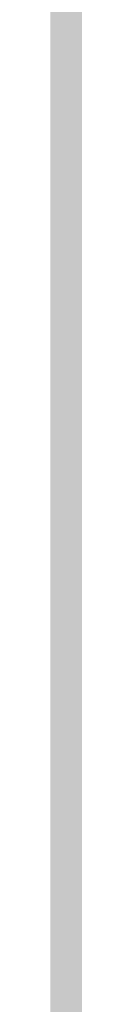
# Model space of a CAD drawing. Units: millimetres. Extents: x 0 to 2267, y 0 to 1823.
# Tile 40 of 256: x 1593.4301 to 1593.4369, y 1226.3857 to 1226.718. Entities that reach past the tile are written whole.
import ezdxf

# ---------------------------------------------------------------- set-up
doc = ezdxf.new("R2010")
doc.units = ezdxf.units.MM
doc.header["$MEASUREMENT"] = 0
doc.layers.add('M-HATC', color=252, linetype='Continuous', lineweight=18)

msp = doc.modelspace()

# ---------------------------------------------------------------- hatches: boundary and pattern name
at = {"layer": 'M-HATC'}
h = msp.add_hatch(color=256, dxfattribs=at)
h.dxf.hatch_style = 1
h.paths.add_polyline_path([(2055.77105, 1603.06204), (1381.08677, 1603.06204), (1381.08677, 1598.06204), (2055.77105, 1598.06204)])
h.paths.add_polyline_path([(2055.77105, 1598.06204), (1381.08677, 1598.06204), (1381.08677, 1593.06204), (2055.77105, 1593.06204)])
h.paths.add_polyline_path([(2051.30737, 1536.76088), (1385.55044, 1536.76088), (1385.55044, 1526.76088), (1387.55044, 1526.76088), (1388.53662, 1525.05276), (1385.33187, 1521.23348), (1385.33187, 1521.22256), (2050.25417, 1522.74913), (2048.32119, 1525.05276), (2049.30737, 1526.76088), (2051.30737, 1526.76088)])
edge = h.paths.add_edge_path()
edge.add_arc((1847.53451, 1379.14917), 135, 222.6030607, 222.8908505, ccw=False)
edge.add_line((1748.16629, 1287.76561), (1683.09212, 1287.76561))
edge.add_arc((1583.7239, 1379.14917), 135, 317.1091495, 317.3969393, ccw=False)
edge.add_arc((1678.9686, 1290.67067), 5, 222.89085, 317.10915, ccw=False)
edge.add_arc((1774.21331, 1379.14917), 135, 222.6030607, 222.8908505, ccw=False)
edge.add_line((1674.84509, 1287.76561), (1609.77092, 1287.76561))
edge.add_arc((1510.4027, 1379.14917), 135, 317.1091495, 317.3969393, ccw=False)
edge.add_arc((1605.6474, 1290.67067), 5, 222.89085, 317.10915, ccw=False)
edge.add_arc((1700.89211, 1379.14917), 135, 222.6030607, 222.8908505, ccw=False)
edge.add_line((1601.52388, 1287.76561), (1536.44972, 1287.76561))
edge.add_arc((1437.08149, 1379.14917), 135, 317.1091495, 317.3969393, ccw=False)
edge.add_arc((1532.3262, 1290.67067), 5, 222.89085, 317.10915, ccw=False)
edge.add_arc((1627.57091, 1379.14917), 135, 222.6030607, 222.8908505, ccw=False)
edge.add_line((1528.20268, 1287.76561), (1505.92891, 1287.76561))
edge.add_spline(control_points=[(1505.92891, 1287.76561), (1504.26224, 1287.76561), (1504.26224, 1282.76561), (1505.92891, 1282.76561)], knot_values=[0, 0, 0, 0, 5, 5, 5, 5], degree=3, periodic=0)
edge.add_line((1505.92891, 1282.76561), (1930.92891, 1282.76561))
edge.add_spline(control_points=[(1930.92891, 1282.76561), (1932.59557, 1282.76561), (1932.59557, 1287.76561), (1930.92891, 1287.76561)], knot_values=[0, 0, 0, 0, 5, 5, 5, 5], degree=3, periodic=0)
edge.add_line((1930.92891, 1287.76561), (1903.05573, 1287.76561))
edge.add_arc((1803.6875, 1379.14917), 135, 317.1091495, 317.3969393, ccw=False)
edge.add_arc((1898.93221, 1290.67067), 5, 222.89085, 317.10915, ccw=False)
edge.add_arc((1994.17691, 1379.14917), 135, 222.6030607, 222.8908505, ccw=False)
edge.add_line((1894.80869, 1287.76561), (1829.73452, 1287.76561))
edge.add_arc((1730.3663, 1379.14917), 135, 317.1091495, 317.3969393, ccw=False)
edge.add_arc((1825.61101, 1290.67067), 5, 222.89085, 317.10915, ccw=False)
edge.add_arc((1920.85571, 1379.14917), 135, 222.6030607, 222.8908505, ccw=False)
edge.add_line((1821.48749, 1287.76561), (1756.41332, 1287.76561))
edge.add_arc((1657.0451, 1379.14917), 135, 317.1091495, 317.3969393, ccw=False)
edge.add_arc((1752.28981, 1290.67067), 5, 222.89085, 317.10915, ccw=False)
edge = h.paths.add_edge_path()
edge.add_spline(control_points=[(1843.42891, 1227.24746), (1845.09557, 1227.24746), (1845.09557, 1232.24746), (1843.42891, 1232.24746)], knot_values=[0, 0, 0, 0, 5, 5, 5, 5], degree=3, periodic=0)
edge.add_line((1843.42891, 1232.24746), (1593.42891, 1232.24746))
edge.add_spline(control_points=[(1593.42891, 1232.24746), (1591.76224, 1232.24746), (1591.76224, 1227.24746), (1593.42891, 1227.24746)], knot_values=[0, 0, 0, 0, 5, 5, 5, 5], degree=3, periodic=0)
edge.add_line((1593.42891, 1227.24746), (1843.42891, 1227.24746))
h.paths.add_polyline_path([(1905.92891, 1127.41706), (1530.92891, 1127.41706, 0.414214), (1520.92891, 1117.41706), (1530.92891, 1117.41706), (1915.92891, 1117.41706, 0.414214)])
edge = h.paths.add_edge_path()
edge.add_arc((1397.08577, 1498.40775), 12.72993, 90.782146, 190.878706, ccw=False)
edge.add_line((1396.912, 1511.13649), (1428.00968, 1511.34875))
edge.add_line((1428.00968, 1511.34875), (1433.00968, 1511.34875))
edge.add_line((1433.00968, 1511.34875), (1434.439, 1511.34875))
edge.add_arc((1419.474, 1498.08041), 20, 41.560995, 74.082109)
edge.add_line((1424.95919, 1517.31353), (1399.93509, 1517.25608))
edge.add_spline(control_points=[(1399.93074, 1517.25607), (1399.88398, 1517.21312), (1399.8328, 1517.16893), (1399.77741, 1517.1236)], knot_values=[11.567499, 11.567499, 11.567499, 11.567499, 11.814249, 11.814249, 11.814249, 11.814249], degree=3, periodic=0)
edge.add_spline(control_points=[(1399.63279, 1517.00986), (1399.58305, 1516.97214), (1399.53072, 1516.93375), (1399.47591, 1516.89474)], knot_values=[11.167718, 11.167718, 11.167718, 11.167718, 11.365188, 11.365188, 11.365188, 11.365188], degree=3, periodic=0)
edge.add_spline(control_points=[(1399.33981, 1516.80007), (1399.15144, 1516.67185), (1398.93836, 1516.5377), (1398.70404, 1516.39942)], knot_values=[10.376405, 10.376405, 10.376405, 10.376405, 11.00994, 11.00994, 11.00994, 11.00994], degree=3, periodic=0)
edge.add_spline(control_points=[(1398.65716, 1516.37187), (1398.57885, 1516.32602), (1398.49825, 1516.27974), (1398.41549, 1516.23309)], knot_values=[10.125175, 10.125175, 10.125175, 10.125175, 10.334406, 10.334406, 10.334406, 10.334406], degree=3, periodic=0)
edge.add_spline(control_points=[(1398.26422, 1516.14874), (1398.19595, 1516.11107), (1398.12634, 1516.07319), (1398.05546, 1516.03513)], knot_values=[9.832246, 9.832246, 9.832246, 9.832246, 9.999658, 9.999658, 9.999658, 9.999658], degree=3, periodic=0)
edge.add_spline(control_points=[(1397.9987, 1516.00476), (1397.73115, 1515.86211), (1397.44602, 1515.71707), (1397.14664, 1515.57138)], knot_values=[9.161808, 9.161808, 9.161808, 9.161808, 9.787769, 9.787769, 9.787769, 9.787769], degree=3, periodic=0)
edge.add_spline(control_points=[(1397.14664, 1515.57138), (1396.84182, 1515.42305), (1396.52223, 1515.27404), (1396.1914, 1515.12621)], knot_values=[8.524455, 8.524455, 8.524455, 8.524455, 9.161808, 9.161808, 9.161808, 9.161808], degree=3, periodic=0)
edge.add_spline(control_points=[(1396.07771, 1515.07565), (1395.98538, 1515.03478), (1395.89222, 1514.99402), (1395.7983, 1514.9534)], knot_values=[8.275193, 8.275193, 8.275193, 8.275193, 8.451726, 8.451726, 8.451726, 8.451726], degree=3, periodic=0)
edge.add_spline(control_points=[(1395.60184, 1514.86912), (1395.49975, 1514.82568), (1395.39685, 1514.78244), (1395.29322, 1514.73944)], knot_values=[7.962917, 7.962917, 7.962917, 7.962917, 8.152764, 8.152764, 8.152764, 8.152764], degree=3, periodic=0)
edge.add_spline(control_points=[(1395.21158, 1514.70568), (1394.82779, 1514.5475), (1394.43452, 1514.39287), (1394.03645, 1514.24422)], knot_values=[7.21254, 7.21254, 7.21254, 7.21254, 7.913148, 7.913148, 7.913148, 7.913148], degree=3, periodic=0)
edge.add_spline(control_points=[(1394.03645, 1514.24422), (1393.70758, 1514.12142), (1393.37544, 1514.0027), (1393.04267, 1513.88945)], knot_values=[6.633733, 6.633733, 6.633733, 6.633733, 7.21254, 7.21254, 7.21254, 7.21254], degree=3, periodic=0)
edge.add_spline(control_points=[(1392.82142, 1513.81499), (1392.71978, 1513.78118), (1392.61815, 1513.74791), (1392.51658, 1513.71521)], knot_values=[6.328796, 6.328796, 6.328796, 6.328796, 6.505493, 6.505493, 6.505493, 6.505493], degree=3, periodic=0)
edge.add_spline(control_points=[(1392.51658, 1513.71521), (1392.31873, 1513.65151), (1392.12116, 1513.59001), (1391.92441, 1513.53098)], knot_values=[5.984605, 5.984605, 5.984605, 5.984605, 6.328796, 6.328796, 6.328796, 6.328796], degree=3, periodic=0)
edge.add_spline(control_points=[(1391.79155, 1513.49146), (1391.31215, 1513.35011), (1390.83842, 1513.22392), (1390.37844, 1513.11711)], knot_values=[5.066697, 5.066697, 5.066697, 5.066697, 5.907055, 5.907055, 5.907055, 5.907055], degree=3, periodic=0)
edge.add_spline(control_points=[(1390.37844, 1513.11711), (1390.17973, 1513.07097), (1389.98359, 1513.02845), (1389.79067, 1512.98988)], knot_values=[4.70367, 4.70367, 4.70367, 4.70367, 5.066695, 5.066695, 5.066695, 5.066695], degree=3, periodic=0)
edge.add_spline(control_points=[(1389.42203, 1512.92036), (1389.24588, 1512.88922), (1389.0729, 1512.86172), (1388.90364, 1512.83814)], knot_values=[4.130571, 4.130571, 4.130571, 4.130571, 4.469816, 4.469816, 4.469816, 4.469816], degree=3, periodic=0)
edge.add_spline(control_points=[(1388.90364, 1512.83814), (1388.59103, 1512.7946), (1388.29108, 1512.76444), (1388.00714, 1512.74941)], knot_values=[3.504031, 3.504031, 3.504031, 3.504031, 4.130571, 4.130571, 4.130571, 4.130571], degree=3, periodic=0)
edge.add_spline(control_points=[(1387.9356, 1512.74593), (1387.85378, 1512.74231), (1387.77334, 1512.73997), (1387.69435, 1512.73898)], knot_values=[3.268866, 3.268866, 3.268866, 3.268866, 3.451164, 3.451164, 3.451164, 3.451164], degree=3, periodic=0)
edge.add_spline(control_points=[(1387.33512, 1512.74426), (1387.20757, 1512.74991), (1387.08472, 1512.7597), (1386.96699, 1512.77385)], knot_values=[2.670686, 2.670686, 2.670686, 2.670686, 2.984, 2.984, 2.984, 2.984], degree=3, periodic=0)
edge.add_spline(control_points=[(1386.83274, 1512.79225), (1386.82093, 1512.79407), (1386.80917, 1512.79594), (1386.79747, 1512.79787)], knot_values=[2.516981, 2.516981, 2.516981, 2.516981, 2.549528, 2.549528, 2.549528, 2.549528], degree=3, periodic=0)
edge.add_spline(control_points=[(1386.45257, 1512.87348), (1386.42573, 1512.88105), (1386.39931, 1512.88895), (1386.3733, 1512.89719)], knot_values=[2.095869, 2.095869, 2.095869, 2.095869, 2.17941, 2.17941, 2.17941, 2.17941], degree=3, periodic=0)
edge.add_spline(control_points=[(1386.06911, 1513.01889), (1386.06338, 1513.02174), (1386.05768, 1513.02463), (1386.05201, 1513.02753)], knot_values=[1.72453, 1.72453, 1.72453, 1.72453, 1.745933, 1.745933, 1.745933, 1.745933], degree=3, periodic=0)
edge.add_arc((1399.474, 1498.08041), 20, 131.824322, 180)
edge.add_arc((1630.33362, 1505.54843), 250.97076, 181.7051759, 236.427975)
edge.add_arc((1605.33992, 1483.30441), 218.7822, 238.660829, 243.3496099)
edge.add_arc((1647.09105, 1510.35917), 262.89859, 183.1298361, 237.8534422, ccw=False)
h.paths.add_polyline_path([(1406.53685, 1391.96444, 0.149382), (1491.55061, 1296.44177, -0.129517)], flags=17)
edge = h.paths.add_edge_path()
edge.add_arc((2037.38381, 1498.08041), 20, 0, 48.265868)
edge.add_spline(control_points=[(2050.69731, 1513.00525), (2050.65121, 1512.98471), (2050.60338, 1512.96554), (2050.55388, 1512.94771)], knot_values=[1.835652, 1.835652, 1.835652, 1.835652, 2.000781, 2.000781, 2.000781, 2.000781], degree=3, periodic=0)
edge.add_spline(control_points=[(2050.46156, 1512.91661), (2050.479, 1512.9221), (2050.49625, 1512.92774), (2050.51332, 1512.93353)], knot_values=[2.045477, 2.045477, 2.045477, 2.045477, 2.101389, 2.101389, 2.101389, 2.101389], degree=3, periodic=0)
edge.add_spline(control_points=[(2050.12896, 1512.83416), (2050.19843, 1512.84734), (2050.26573, 1512.86233), (2050.33075, 1512.87919)], knot_values=[2.237629, 2.237629, 2.237629, 2.237629, 2.435841, 2.435841, 2.435841, 2.435841], degree=3, periodic=0)
edge.add_spline(control_points=[(2050.09463, 1512.82783), (2050.10613, 1512.82989), (2050.11757, 1512.832), (2050.12896, 1512.83416)], knot_values=[2.435841, 2.435841, 2.435841, 2.435841, 2.468321, 2.468321, 2.468321, 2.468321], degree=3, periodic=0)
edge.add_spline(control_points=[(2049.78433, 1512.78511), (2049.85521, 1512.79219), (2049.92435, 1512.80077), (2049.99166, 1512.81088)], knot_values=[2.563852, 2.563852, 2.563852, 2.563852, 2.748541, 2.748541, 2.748541, 2.748541], degree=3, periodic=0)
edge.add_spline(control_points=[(2049.4052, 1512.76169), (2049.5364, 1512.76526), (2049.66292, 1512.77299), (2049.78433, 1512.78511)], knot_values=[2.748541, 2.748541, 2.748541, 2.748541, 3.064882, 3.064882, 3.064882, 3.064882], degree=3, periodic=0)
edge.add_spline(control_points=[(2049.16976, 1512.75968), (2049.23364, 1512.7591), (2049.29654, 1512.7594), (2049.35844, 1512.7606)], knot_values=[3.102309, 3.102309, 3.102309, 3.102309, 3.2503, 3.2503, 3.2503, 3.2503], degree=3, periodic=0)
edge.add_spline(control_points=[(2048.85727, 1512.76911), (2048.96378, 1512.76378), (2049.068, 1512.76061), (2049.16976, 1512.75968)], knot_values=[3.2503, 3.2503, 3.2503, 3.2503, 3.486069, 3.486069, 3.486069, 3.486069], degree=3, periodic=0)
edge.add_spline(control_points=[(2048.69241, 1512.77892), (2048.3729, 1512.80093), (2048.0345, 1512.84106), (2047.68175, 1512.89697)], knot_values=[3.606429, 3.606429, 3.606429, 3.606429, 4.2989, 4.2989, 4.2989, 4.2989], degree=3, periodic=0)
edge.add_spline(control_points=[(2047.68175, 1512.89697), (2047.5458, 1512.91852), (2047.40772, 1512.94241), (2047.26776, 1512.96851)], knot_values=[4.2989, 4.2989, 4.2989, 4.2989, 4.565769, 4.565769, 4.565769, 4.565769], degree=3, periodic=0)
edge.add_spline(control_points=[(2047.26776, 1512.96851), (2047.14494, 1512.99141), (2047.02067, 1513.01601), (2046.89514, 1513.04223)], knot_values=[4.565769, 4.565769, 4.565769, 4.565769, 4.799971, 4.799971, 4.799971, 4.799971], degree=3, periodic=0)
edge.add_spline(control_points=[(2046.89514, 1513.04223), (2046.52865, 1513.11875), (2046.15135, 1513.20899), (2045.7676, 1513.31068)], knot_values=[4.799971, 4.799971, 4.799971, 4.799971, 5.483718, 5.483718, 5.483718, 5.483718], degree=3, periodic=0)
edge.add_spline(control_points=[(2045.7676, 1513.31068), (2045.3724, 1513.41539), (2044.97036, 1513.53225), (2044.56625, 1513.65876)], knot_values=[5.483718, 5.483718, 5.483718, 5.483718, 6.187866, 6.187866, 6.187866, 6.187866], degree=3, periodic=0)
edge.add_spline(control_points=[(2044.56625, 1513.65876), (2044.41491, 1513.70614), (2044.26329, 1513.75487), (2044.11163, 1513.80482)], knot_values=[6.187866, 6.187866, 6.187866, 6.187866, 6.451551, 6.451551, 6.451551, 6.451551], degree=3, periodic=0)
edge.add_spline(control_points=[(2044.11163, 1513.80482), (2043.99666, 1513.84269), (2043.88167, 1513.88126), (2043.76676, 1513.92048)], knot_values=[6.451551, 6.451551, 6.451551, 6.451551, 6.651434, 6.651434, 6.651434, 6.651434], degree=3, periodic=0)
edge.add_spline(control_points=[(2043.76676, 1513.92048), (2043.37157, 1514.05536), (2042.97738, 1514.19789), (2042.58863, 1514.34575)], knot_values=[6.651434, 6.651434, 6.651434, 6.651434, 7.338879, 7.338879, 7.338879, 7.338879], degree=3, periodic=0)
edge.add_spline(control_points=[(2042.58863, 1514.34575), (2042.16431, 1514.50715), (2041.74647, 1514.67491), (2041.34086, 1514.84603)], knot_values=[7.338879, 7.338879, 7.338879, 7.338879, 8.089209, 8.089209, 8.089209, 8.089209], degree=3, periodic=0)
edge.add_spline(control_points=[(2041.34086, 1514.84603), (2041.1028, 1514.94647), (2040.86896, 1515.04806), (2040.64049, 1515.1502)], knot_values=[8.089209, 8.089209, 8.089209, 8.089209, 8.529587, 8.529587, 8.529587, 8.529587], degree=3, periodic=0)
edge.add_spline(control_points=[(2040.50999, 1515.20887), (2040.08238, 1515.40218), (2039.67475, 1515.59705), (2039.29495, 1515.78939)], knot_values=[8.613818, 8.613818, 8.613818, 8.613818, 9.44571, 9.44571, 9.44571, 9.44571], degree=3, periodic=0)
edge.add_spline(control_points=[(2039.29495, 1515.78939), (2039.0618, 1515.90746), (2038.83914, 1516.02458), (2038.62878, 1516.1398)], knot_values=[9.44571, 9.44571, 9.44571, 9.44571, 9.956404, 9.956404, 9.956404, 9.956404], degree=3, periodic=0)
edge.add_spline(control_points=[(2038.62878, 1516.1398), (2038.51874, 1516.20007), (2038.41207, 1516.25982), (2038.30903, 1516.31891)], knot_values=[9.956404, 9.956404, 9.956404, 9.956404, 10.223542, 10.223542, 10.223542, 10.223542], degree=3, periodic=0)
edge.add_spline(control_points=[(2038.30903, 1516.31891), (2038.21377, 1516.37354), (2038.12161, 1516.42762), (2038.03275, 1516.48102)], knot_values=[10.223542, 10.223542, 10.223542, 10.223542, 10.47051, 10.47051, 10.47051, 10.47051], degree=3, periodic=0)
edge.add_spline(control_points=[(2038.03275, 1516.48102), (2037.78552, 1516.62961), (2037.56388, 1516.77304), (2037.37225, 1516.909)], knot_values=[10.47051, 10.47051, 10.47051, 10.47051, 11.15767, 11.15767, 11.15767, 11.15767], degree=3, periodic=0)
edge.add_spline(control_points=[(2037.37225, 1516.909), (2037.27893, 1516.9752), (2037.19274, 1517.03963), (2037.11417, 1517.10203)], knot_values=[11.15767, 11.15767, 11.15767, 11.15767, 11.49227, 11.49227, 11.49227, 11.49227], degree=3, periodic=0)
edge.add_spline(control_points=[(2036.85638, 1517.32585), (2036.91481, 1517.26923), (2036.98143, 1517.21027), (2037.05573, 1517.14922)], knot_values=[11.577341, 11.577341, 11.577341, 11.577341, 11.91035, 11.91035, 11.91035, 11.91035], degree=3, periodic=0)
edge.add_spline(control_points=[(2036.80739, 1517.37475), (2036.82301, 1517.35865), (2036.83935, 1517.34235), (2036.85638, 1517.32585)], knot_values=[11.91035, 11.91035, 11.91035, 11.91035, 12.007402, 12.007402, 12.007402, 12.007402], degree=3, periodic=0)
edge.add_spline(control_points=[(2036.70167, 1517.494), (2036.71042, 1517.48299), (2036.71958, 1517.47185), (2036.72913, 1517.4606)], knot_values=[12.184155, 12.184155, 12.184155, 12.184155, 12.255409, 12.255409, 12.255409, 12.255409], degree=3, periodic=0)
edge.add_spline(control_points=[(2036.6159, 1517.6205), (2036.61998, 1517.61304), (2036.6243, 1517.6055), (2036.62885, 1517.59789)], knot_values=[12.487913, 12.487913, 12.487913, 12.487913, 12.541035, 12.541035, 12.541035, 12.541035], degree=3, periodic=0)
edge.add_spline(control_points=[(2036.56349, 1517.78599), (2036.56372, 1517.77936), (2036.56423, 1517.77264), (2036.56502, 1517.76582)], knot_values=[12.911761, 12.911761, 12.911761, 12.911761, 12.968286, 12.968286, 12.968286, 12.968286], degree=3, periodic=0)
edge.add_spline(control_points=[(2036.61663, 1517.93042), (2036.61248, 1517.92586), (2036.60857, 1517.92121), (2036.60491, 1517.91648)], knot_values=[13.382527, 13.382527, 13.382527, 13.382527, 13.433791, 13.433791, 13.433791, 13.433791], degree=3, periodic=0)
edge.add_spline(control_points=[(2036.74902, 1518.01695), (2036.73613, 1518.0116), (2036.72393, 1518.00601), (2036.71242, 1518.00018)], knot_values=[13.726299, 13.726299, 13.726299, 13.726299, 13.809928, 13.809928, 13.809928, 13.809928], degree=3, periodic=0)
edge.add_spline(control_points=[(2036.86043, 1518.05285), (2036.83863, 1518.04743), (2036.81809, 1518.04156), (2036.79879, 1518.03526)], knot_values=[13.910887, 13.910887, 13.910887, 13.910887, 14.02153, 14.02153, 14.02153, 14.02153], degree=3, periodic=0)
edge.add_line((2036.96387, 1518.08041), (2032.38381, 1518.08041))
edge.add_line((2032.38381, 1518.08041), (2027.38381, 1518.08041))
edge.add_line((2027.38381, 1518.08041), (2022.38381, 1518.08041))
edge.add_line((2022.38381, 1518.08041), (2017.38381, 1518.08041))
edge.add_arc((2017.38381, 1498.08041), 20, 90, 138.439005)
edge.add_line((2002.41881, 1511.34875), (2003.84813, 1511.34875))
edge.add_line((2003.84813, 1511.34875), (2008.84813, 1511.34875))
edge.add_line((2008.84813, 1511.34875), (2039.77204, 1511.13768))
edge.add_arc((2039.77204, 1498.40775), 12.72993, -10.878706, 90, ccw=False)
edge.add_arc((1789.76676, 1510.35917), 262.89859, 302.1465578, 356.8701639, ccw=False)
edge.add_arc((1831.51789, 1483.30441), 218.7822, 296.6503901, 301.339171)
edge.add_arc((1806.52419, 1505.54843), 250.97076, 303.572025, 358.2948241)
h.paths.add_polyline_path([(2030.32096, 1391.96444, -0.129517), (1945.3072, 1296.44177, 0.149382)], flags=17)
edge = h.paths.add_edge_path()
edge.add_spline(control_points=[(2037.2464, 1518.08209), (2037.28977, 1518.08098), (2037.33555, 1518.08041), (2037.3838, 1518.08041)], knot_values=[0.000012, 0.000012, 0.000012, 0.000012, 0.144754, 0.144754, 0.144754, 0.144754], degree=3, periodic=0)
edge.add_line((2037.33571, 1518.08041), (2037.00963, 1518.08041))
edge.add_spline(control_points=[(2037.00963, 1518.08041), (2036.98217, 1518.07678), (2036.95605, 1518.07266), (2036.93124, 1518.06808)], knot_values=[14.13465, 14.13465, 14.13465, 14.13465, 14.247197, 14.247197, 14.247197, 14.247197], degree=3, periodic=0)
edge.add_spline(control_points=[(2036.93124, 1518.06808), (2036.92764, 1518.06741), (2036.92407, 1518.06674), (2036.92053, 1518.06605)], knot_values=[14.118315, 14.118315, 14.118315, 14.118315, 14.13465, 14.13465, 14.13465, 14.13465], degree=3, periodic=0)
edge.add_spline(control_points=[(2036.92053, 1518.06605), (2036.9118, 1518.06436), (2036.90323, 1518.06262), (2036.89484, 1518.06081)], knot_values=[14.078086, 14.078086, 14.078086, 14.078086, 14.118315, 14.118315, 14.118315, 14.118315], degree=3, periodic=0)
edge.add_spline(control_points=[(2036.89484, 1518.06081), (2036.88304, 1518.05827), (2036.87157, 1518.05562), (2036.86043, 1518.05285)], knot_values=[14.02153, 14.02153, 14.02153, 14.02153, 14.078086, 14.078086, 14.078086, 14.078086], degree=3, periodic=0)
edge.add_spline(control_points=[(2036.86043, 1518.05285), (2036.83863, 1518.04743), (2036.81809, 1518.04156), (2036.79879, 1518.03526)], knot_values=[13.910887, 13.910887, 13.910887, 13.910887, 14.02153, 14.02153, 14.02153, 14.02153], degree=3, periodic=0)
edge.add_spline(control_points=[(2036.79879, 1518.03526), (2036.79809, 1518.03504), (2036.7974, 1518.03481), (2036.79671, 1518.03458)], knot_values=[13.906906, 13.906906, 13.906906, 13.906906, 13.910887, 13.910887, 13.910887, 13.910887], degree=3, periodic=0)
edge.add_spline(control_points=[(2036.79671, 1518.03458), (2036.78819, 1518.03178), (2036.77991, 1518.02888), (2036.77187, 1518.02591)], knot_values=[13.857826, 13.857826, 13.857826, 13.857826, 13.906906, 13.906906, 13.906906, 13.906906], degree=3, periodic=0)
edge.add_spline(control_points=[(2036.77187, 1518.02591), (2036.76402, 1518.023), (2036.75641, 1518.02002), (2036.74902, 1518.01695)], knot_values=[13.809928, 13.809928, 13.809928, 13.809928, 13.857826, 13.857826, 13.857826, 13.857826], degree=3, periodic=0)
edge.add_spline(control_points=[(2036.74902, 1518.01695), (2036.73613, 1518.0116), (2036.72393, 1518.00601), (2036.71242, 1518.00018)], knot_values=[13.726299, 13.726299, 13.726299, 13.726299, 13.809928, 13.809928, 13.809928, 13.809928], degree=3, periodic=0)
edge.add_spline(control_points=[(2036.71242, 1518.00018), (2036.71211, 1518.00002), (2036.71179, 1517.99986), (2036.71147, 1517.99969)], knot_values=[13.723993, 13.723993, 13.723993, 13.723993, 13.726299, 13.726299, 13.726299, 13.726299], degree=3, periodic=0)
edge.add_spline(control_points=[(2036.71147, 1517.99969), (2036.70634, 1517.99708), (2036.70134, 1517.99441), (2036.69648, 1517.9917)], knot_values=[13.686536, 13.686536, 13.686536, 13.686536, 13.723993, 13.723993, 13.723993, 13.723993], degree=3, periodic=0)
edge.add_spline(control_points=[(2036.69648, 1517.9917), (2036.6919, 1517.98914), (2036.68744, 1517.98654), (2036.6831, 1517.9839)], knot_values=[13.651251, 13.651251, 13.651251, 13.651251, 13.686536, 13.686536, 13.686536, 13.686536], degree=3, periodic=0)
edge.add_spline(control_points=[(2036.6831, 1517.9839), (2036.67641, 1517.97983), (2036.67001, 1517.97566), (2036.6639, 1517.97139)], knot_values=[13.596804, 13.596804, 13.596804, 13.596804, 13.651251, 13.651251, 13.651251, 13.651251], degree=3, periodic=0)
edge.add_spline(control_points=[(2036.6639, 1517.97139), (2036.66358, 1517.97117), (2036.66326, 1517.97094), (2036.66294, 1517.97072)], knot_values=[13.593956, 13.593956, 13.593956, 13.593956, 13.596804, 13.596804, 13.596804, 13.596804], degree=3, periodic=0)
edge.add_spline(control_points=[(2036.66294, 1517.97072), (2036.6603, 1517.96886), (2036.65771, 1517.96698), (2036.65518, 1517.96509)], knot_values=[13.570322, 13.570322, 13.570322, 13.570322, 13.593956, 13.593956, 13.593956, 13.593956], degree=3, periodic=0)
edge.add_spline(control_points=[(2036.65518, 1517.96509), (2036.65251, 1517.9631), (2036.64991, 1517.96108), (2036.64737, 1517.95905)], knot_values=[13.545477, 13.545477, 13.545477, 13.545477, 13.570322, 13.570322, 13.570322, 13.570322], degree=3, periodic=0)
edge.add_spline(control_points=[(2036.64737, 1517.95905), (2036.64721, 1517.95892), (2036.64705, 1517.9588), (2036.64689, 1517.95867)], knot_values=[13.543931, 13.543931, 13.543931, 13.543931, 13.545477, 13.545477, 13.545477, 13.545477], degree=3, periodic=0)
edge.add_spline(control_points=[(2036.64689, 1517.95867), (2036.64121, 1517.95411), (2036.63582, 1517.94945), (2036.63073, 1517.94468)], knot_values=[13.488237, 13.488237, 13.488237, 13.488237, 13.543931, 13.543931, 13.543931, 13.543931], degree=3, periodic=0)
edge.add_spline(control_points=[(2036.63073, 1517.94468), (2036.62817, 1517.94229), (2036.62569, 1517.93988), (2036.62329, 1517.93744)], knot_values=[13.460307, 13.460307, 13.460307, 13.460307, 13.488237, 13.488237, 13.488237, 13.488237], degree=3, periodic=0)
edge.add_spline(control_points=[(2036.62329, 1517.93744), (2036.62151, 1517.93564), (2036.61978, 1517.93383), (2036.61809, 1517.932)], knot_values=[13.439712, 13.439712, 13.439712, 13.439712, 13.460307, 13.460307, 13.460307, 13.460307], degree=3, periodic=0)
edge.add_spline(control_points=[(2036.61809, 1517.932), (2036.6176, 1517.93147), (2036.61711, 1517.93095), (2036.61663, 1517.93042)], knot_values=[13.433791, 13.433791, 13.433791, 13.433791, 13.439712, 13.439712, 13.439712, 13.439712], degree=3, periodic=0)
edge.add_spline(control_points=[(2036.61663, 1517.93042), (2036.61248, 1517.92586), (2036.60857, 1517.92121), (2036.60491, 1517.91648)], knot_values=[13.382527, 13.382527, 13.382527, 13.382527, 13.433791, 13.433791, 13.433791, 13.433791], degree=3, periodic=0)
edge.add_spline(control_points=[(2036.60491, 1517.91648), (2036.60258, 1517.91347), (2036.60036, 1517.91044), (2036.59824, 1517.90737)], knot_values=[13.350017, 13.350017, 13.350017, 13.350017, 13.382527, 13.382527, 13.382527, 13.382527], degree=3, periodic=0)
edge.add_spline(control_points=[(2036.59824, 1517.90737), (2036.59718, 1517.90585), (2036.59616, 1517.90433), (2036.59515, 1517.90279)], knot_values=[13.333922, 13.333922, 13.333922, 13.333922, 13.350017, 13.350017, 13.350017, 13.350017], degree=3, periodic=0)
edge.add_spline(control_points=[(2036.59515, 1517.90279), (2036.59452, 1517.90183), (2036.5939, 1517.90086), (2036.59329, 1517.89989)], knot_values=[13.323828, 13.323828, 13.323828, 13.323828, 13.333922, 13.333922, 13.333922, 13.333922], degree=3, periodic=0)
edge.add_spline(control_points=[(2036.59329, 1517.89989), (2036.59049, 1517.89545), (2036.5879, 1517.89094), (2036.5855, 1517.88637)], knot_values=[13.277545, 13.277545, 13.277545, 13.277545, 13.323828, 13.323828, 13.323828, 13.323828], degree=3, periodic=0)
edge.add_spline(control_points=[(2036.5855, 1517.88637), (2036.58355, 1517.88267), (2036.58174, 1517.87892), (2036.58006, 1517.87513)], knot_values=[13.240119, 13.240119, 13.240119, 13.240119, 13.277545, 13.277545, 13.277545, 13.277545], degree=3, periodic=0)
edge.add_spline(control_points=[(2036.58006, 1517.87513), (2036.57952, 1517.87393), (2036.579, 1517.87272), (2036.57849, 1517.87151)], knot_values=[13.228211, 13.228211, 13.228211, 13.228211, 13.240119, 13.240119, 13.240119, 13.240119], degree=3, periodic=0)
edge.add_spline(control_points=[(2036.57849, 1517.87151), (2036.57796, 1517.87023), (2036.57744, 1517.86896), (2036.57693, 1517.86767)], knot_values=[13.215717, 13.215717, 13.215717, 13.215717, 13.228211, 13.228211, 13.228211, 13.228211], degree=3, periodic=0)
edge.add_spline(control_points=[(2036.57693, 1517.86767), (2036.57548, 1517.86399), (2036.57414, 1517.86027), (2036.57293, 1517.85651)], knot_values=[13.179847, 13.179847, 13.179847, 13.179847, 13.215717, 13.215717, 13.215717, 13.215717], degree=3, periodic=0)
edge.add_spline(control_points=[(2036.57293, 1517.85651), (2036.5713, 1517.8515), (2036.56989, 1517.84641), (2036.56868, 1517.84126)], knot_values=[13.132017, 13.132017, 13.132017, 13.132017, 13.179847, 13.179847, 13.179847, 13.179847], degree=3, periodic=0)
edge.add_spline(control_points=[(2036.56868, 1517.84126), (2036.56844, 1517.84023), (2036.56821, 1517.8392), (2036.56798, 1517.83817)], knot_values=[13.122482, 13.122482, 13.122482, 13.122482, 13.132017, 13.132017, 13.132017, 13.132017], degree=3, periodic=0)
edge.add_spline(control_points=[(2036.56798, 1517.83817), (2036.56758, 1517.83634), (2036.56721, 1517.8345), (2036.56687, 1517.83266)], knot_values=[13.105592, 13.105592, 13.105592, 13.105592, 13.122482, 13.122482, 13.122482, 13.122482], degree=3, periodic=0)
edge.add_spline(control_points=[(2036.56687, 1517.83266), (2036.56622, 1517.82921), (2036.56567, 1517.82574), (2036.5652, 1517.82223)], knot_values=[13.074063, 13.074063, 13.074063, 13.074063, 13.105592, 13.105592, 13.105592, 13.105592], degree=3, periodic=0)
edge.add_spline(control_points=[(2036.5652, 1517.82223), (2036.5652, 1517.82223), (2036.5652, 1517.82223), (2036.5652, 1517.82223)], knot_values=[13.074043, 13.074043, 13.074043, 13.074043, 13.074063, 13.074063, 13.074063, 13.074063], degree=3, periodic=0)
edge.add_spline(control_points=[(2036.5652, 1517.82223), (2036.56443, 1517.81643), (2036.5639, 1517.81055), (2036.56361, 1517.8046)], knot_values=[13.021884, 13.021884, 13.021884, 13.021884, 13.074043, 13.074043, 13.074043, 13.074043], degree=3, periodic=0)
edge.add_spline(control_points=[(2036.56361, 1517.8046), (2036.56358, 1517.80401), (2036.56356, 1517.80342), (2036.56353, 1517.80283)], knot_values=[13.01674, 13.01674, 13.01674, 13.01674, 13.021884, 13.021884, 13.021884, 13.021884], degree=3, periodic=0)
edge.add_spline(control_points=[(2036.56353, 1517.80283), (2036.56344, 1517.80051), (2036.56338, 1517.79817), (2036.56336, 1517.79582)], knot_values=[12.996438, 12.996438, 12.996438, 12.996438, 13.01674, 13.01674, 13.01674, 13.01674], degree=3, periodic=0)
edge.add_spline(control_points=[(2036.56336, 1517.79582), (2036.56334, 1517.79257), (2036.56338, 1517.78929), (2036.56349, 1517.78599)], knot_values=[12.968286, 12.968286, 12.968286, 12.968286, 12.996438, 12.996438, 12.996438, 12.996438], degree=3, periodic=0)
edge.add_spline(control_points=[(2036.56349, 1517.78599), (2036.56372, 1517.77936), (2036.56423, 1517.77264), (2036.56502, 1517.76582)], knot_values=[12.911761, 12.911761, 12.911761, 12.911761, 12.968286, 12.968286, 12.968286, 12.968286], degree=3, periodic=0)
edge.add_spline(control_points=[(2036.56502, 1517.76582), (2036.56503, 1517.76573), (2036.56504, 1517.76564), (2036.56505, 1517.76555)], knot_values=[12.911017, 12.911017, 12.911017, 12.911017, 12.911761, 12.911761, 12.911761, 12.911761], degree=3, periodic=0)
edge.add_spline(control_points=[(2036.56505, 1517.76555), (2036.56541, 1517.76245), (2036.56583, 1517.75933), (2036.56631, 1517.75619)], knot_values=[12.88528, 12.88528, 12.88528, 12.88528, 12.911017, 12.911017, 12.911017, 12.911017], degree=3, periodic=0)
edge.add_spline(control_points=[(2036.56631, 1517.75619), (2036.56673, 1517.75341), (2036.5672, 1517.75062), (2036.56771, 1517.74782)], knot_values=[12.862519, 12.862519, 12.862519, 12.862519, 12.88528, 12.88528, 12.88528, 12.88528], degree=3, periodic=0)
edge.add_spline(control_points=[(2036.56771, 1517.74782), (2036.56779, 1517.74737), (2036.56788, 1517.74692), (2036.56796, 1517.74647)], knot_values=[12.858885, 12.858885, 12.858885, 12.858885, 12.862519, 12.862519, 12.862519, 12.862519], degree=3, periodic=0)
edge.add_spline(control_points=[(2036.56796, 1517.74647), (2036.5692, 1517.73986), (2036.57069, 1517.73316), (2036.57243, 1517.72638)], knot_values=[12.8053, 12.8053, 12.8053, 12.8053, 12.858885, 12.858885, 12.858885, 12.858885], degree=3, periodic=0)
edge.add_spline(control_points=[(2036.57243, 1517.72638), (2036.5734, 1517.72257), (2036.57446, 1517.71874), (2036.57559, 1517.71488)], knot_values=[12.775176, 12.775176, 12.775176, 12.775176, 12.8053, 12.8053, 12.8053, 12.8053], degree=3, periodic=0)
edge.add_spline(control_points=[(2036.57559, 1517.71488), (2036.57628, 1517.71252), (2036.577, 1517.71015), (2036.57775, 1517.70778)], knot_values=[12.756759, 12.756759, 12.756759, 12.756759, 12.775176, 12.775176, 12.775176, 12.775176], degree=3, periodic=0)
edge.add_spline(control_points=[(2036.57775, 1517.70778), (2036.57808, 1517.70674), (2036.57841, 1517.7057), (2036.57875, 1517.70466)], knot_values=[12.748742, 12.748742, 12.748742, 12.748742, 12.756759, 12.756759, 12.756759, 12.756759], degree=3, periodic=0)
edge.add_spline(control_points=[(2036.57875, 1517.70466), (2036.58082, 1517.6983), (2036.58309, 1517.69187), (2036.58557, 1517.68537)], knot_values=[12.69959, 12.69959, 12.69959, 12.69959, 12.748742, 12.748742, 12.748742, 12.748742], degree=3, periodic=0)
edge.add_spline(control_points=[(2036.58557, 1517.68537), (2036.58762, 1517.68001), (2036.5898, 1517.6746), (2036.59213, 1517.66916)], knot_values=[12.659038, 12.659038, 12.659038, 12.659038, 12.69959, 12.69959, 12.69959, 12.69959], degree=3, periodic=0)
edge.add_spline(control_points=[(2036.59213, 1517.66916), (2036.59397, 1517.66482), (2036.59591, 1517.66047), (2036.59793, 1517.65608)], knot_values=[12.626806, 12.626806, 12.626806, 12.626806, 12.659038, 12.659038, 12.659038, 12.659038], degree=3, periodic=0)
edge.add_spline(control_points=[(2036.59793, 1517.65608), (2036.59839, 1517.65507), (2036.59886, 1517.65406), (2036.59934, 1517.65305)], knot_values=[12.619394, 12.619394, 12.619394, 12.619394, 12.626806, 12.626806, 12.626806, 12.626806], degree=3, periodic=0)
edge.add_spline(control_points=[(2036.59934, 1517.65305), (2036.60435, 1517.64236), (2036.60987, 1517.63151), (2036.61589, 1517.6205)], knot_values=[12.541039, 12.541039, 12.541039, 12.541039, 12.619394, 12.619394, 12.619394, 12.619394], degree=3, periodic=0)
edge.add_spline(control_points=[(2036.61589, 1517.6205), (2036.61589, 1517.6205), (2036.6159, 1517.6205), (2036.6159, 1517.6205)], knot_values=[12.541035, 12.541035, 12.541035, 12.541035, 12.541039, 12.541039, 12.541039, 12.541039], degree=3, periodic=0)
edge.add_spline(control_points=[(2036.6159, 1517.6205), (2036.61998, 1517.61304), (2036.6243, 1517.6055), (2036.62885, 1517.59789)], knot_values=[12.487913, 12.487913, 12.487913, 12.487913, 12.541035, 12.541035, 12.541035, 12.541035], degree=3, periodic=0)
edge.add_spline(control_points=[(2036.62885, 1517.59789), (2036.63261, 1517.5916), (2036.63653, 1517.58526), (2036.64061, 1517.57888)], knot_values=[12.443982, 12.443982, 12.443982, 12.443982, 12.487913, 12.487913, 12.487913, 12.487913], degree=3, periodic=0)
edge.add_spline(control_points=[(2036.64061, 1517.57888), (2036.64144, 1517.57757), (2036.64228, 1517.57626), (2036.64313, 1517.57495)], knot_values=[12.434996, 12.434996, 12.434996, 12.434996, 12.443982, 12.443982, 12.443982, 12.443982], degree=3, periodic=0)
edge.add_spline(control_points=[(2036.64313, 1517.57495), (2036.65306, 1517.55958), (2036.66389, 1517.54394), (2036.6756, 1517.52803)], knot_values=[12.329647, 12.329647, 12.329647, 12.329647, 12.434996, 12.434996, 12.434996, 12.434996], degree=3, periodic=0)
edge.add_spline(control_points=[(2036.6756, 1517.52803), (2036.68385, 1517.51682), (2036.69254, 1517.50548), (2036.70167, 1517.494)], knot_values=[12.255409, 12.255409, 12.255409, 12.255409, 12.329647, 12.329647, 12.329647, 12.329647], degree=3, periodic=0)
edge.add_spline(control_points=[(2036.70167, 1517.494), (2036.71042, 1517.48299), (2036.71958, 1517.47185), (2036.72913, 1517.4606)], knot_values=[12.184155, 12.184155, 12.184155, 12.184155, 12.255409, 12.255409, 12.255409, 12.255409], degree=3, periodic=0)
edge.add_spline(control_points=[(2036.72913, 1517.4606), (2036.74363, 1517.44352), (2036.75904, 1517.42617), (2036.77534, 1517.40855)], knot_values=[12.075961, 12.075961, 12.075961, 12.075961, 12.184155, 12.184155, 12.184155, 12.184155], degree=3, periodic=0)
edge.add_spline(control_points=[(2036.77534, 1517.40855), (2036.77631, 1517.4075), (2036.77729, 1517.40645), (2036.77827, 1517.40539)], knot_values=[12.069502, 12.069502, 12.069502, 12.069502, 12.075961, 12.075961, 12.075961, 12.075961], degree=3, periodic=0)
edge.add_spline(control_points=[(2036.77827, 1517.40539), (2036.78768, 1517.39526), (2036.79739, 1517.38505), (2036.80739, 1517.37475)], knot_values=[12.007402, 12.007402, 12.007402, 12.007402, 12.069502, 12.069502, 12.069502, 12.069502], degree=3, periodic=0)
edge.add_spline(control_points=[(2036.80739, 1517.37475), (2036.82301, 1517.35865), (2036.83935, 1517.34235), (2036.85638, 1517.32585)], knot_values=[11.91035, 11.91035, 11.91035, 11.91035, 12.007402, 12.007402, 12.007402, 12.007402], degree=3, periodic=0)
edge.add_spline(control_points=[(2036.85638, 1517.32585), (2036.91481, 1517.26923), (2036.98143, 1517.21027), (2037.05573, 1517.14922)], knot_values=[11.577341, 11.577341, 11.577341, 11.577341, 11.91035, 11.91035, 11.91035, 11.91035], degree=3, periodic=0)
edge.add_spline(control_points=[(2037.05573, 1517.14922), (2037.07471, 1517.13362), (2037.0942, 1517.11789), (2037.11417, 1517.10203)], knot_values=[11.49227, 11.49227, 11.49227, 11.49227, 11.577341, 11.577341, 11.577341, 11.577341], degree=3, periodic=0)
edge.add_spline(control_points=[(2037.11417, 1517.10203), (2037.19274, 1517.03963), (2037.27893, 1516.9752), (2037.37225, 1516.909)], knot_values=[11.15767, 11.15767, 11.15767, 11.15767, 11.49227, 11.49227, 11.49227, 11.49227], degree=3, periodic=0)
edge.add_spline(control_points=[(2037.37225, 1516.909), (2037.56388, 1516.77304), (2037.78552, 1516.62961), (2038.03275, 1516.48102)], knot_values=[10.47051, 10.47051, 10.47051, 10.47051, 11.15767, 11.15767, 11.15767, 11.15767], degree=3, periodic=0)
edge.add_spline(control_points=[(2038.03275, 1516.48102), (2038.12161, 1516.42762), (2038.21377, 1516.37354), (2038.30903, 1516.31891)], knot_values=[10.223542, 10.223542, 10.223542, 10.223542, 10.47051, 10.47051, 10.47051, 10.47051], degree=3, periodic=0)
edge.add_spline(control_points=[(2038.30903, 1516.31891), (2038.41207, 1516.25982), (2038.51874, 1516.20007), (2038.62878, 1516.1398)], knot_values=[9.956404, 9.956404, 9.956404, 9.956404, 10.223542, 10.223542, 10.223542, 10.223542], degree=3, periodic=0)
edge.add_spline(control_points=[(2038.62878, 1516.1398), (2038.83914, 1516.02458), (2039.0618, 1515.90746), (2039.29495, 1515.78939)], knot_values=[9.44571, 9.44571, 9.44571, 9.44571, 9.956404, 9.956404, 9.956404, 9.956404], degree=3, periodic=0)
edge.add_spline(control_points=[(2039.29495, 1515.78939), (2039.67475, 1515.59705), (2040.08238, 1515.40218), (2040.50999, 1515.20887)], knot_values=[8.613818, 8.613818, 8.613818, 8.613818, 9.44571, 9.44571, 9.44571, 9.44571], degree=3, periodic=0)
edge.add_spline(control_points=[(2040.50999, 1515.20887), (2040.55329, 1515.1893), (2040.59679, 1515.16974), (2040.64049, 1515.1502)], knot_values=[8.529587, 8.529587, 8.529587, 8.529587, 8.613818, 8.613818, 8.613818, 8.613818], degree=3, periodic=0)
edge.add_spline(control_points=[(2040.64049, 1515.1502), (2040.86896, 1515.04806), (2041.1028, 1514.94647), (2041.34086, 1514.84603)], knot_values=[8.089209, 8.089209, 8.089209, 8.089209, 8.529587, 8.529587, 8.529587, 8.529587], degree=3, periodic=0)
edge.add_spline(control_points=[(2041.34086, 1514.84603), (2041.74647, 1514.67491), (2042.16431, 1514.50715), (2042.58863, 1514.34575)], knot_values=[7.338879, 7.338879, 7.338879, 7.338879, 8.089209, 8.089209, 8.089209, 8.089209], degree=3, periodic=0)
edge.add_spline(control_points=[(2042.58863, 1514.34575), (2042.97738, 1514.19789), (2043.37157, 1514.05536), (2043.76676, 1513.92048)], knot_values=[6.651434, 6.651434, 6.651434, 6.651434, 7.338879, 7.338879, 7.338879, 7.338879], degree=3, periodic=0)
edge.add_spline(control_points=[(2043.76676, 1513.92048), (2043.88167, 1513.88126), (2043.99666, 1513.84269), (2044.11163, 1513.80482)], knot_values=[6.451551, 6.451551, 6.451551, 6.451551, 6.651434, 6.651434, 6.651434, 6.651434], degree=3, periodic=0)
edge.add_spline(control_points=[(2044.11163, 1513.80482), (2044.26329, 1513.75487), (2044.41491, 1513.70614), (2044.56625, 1513.65876)], knot_values=[6.187866, 6.187866, 6.187866, 6.187866, 6.451551, 6.451551, 6.451551, 6.451551], degree=3, periodic=0)
edge.add_spline(control_points=[(2044.56625, 1513.65876), (2044.97036, 1513.53225), (2045.3724, 1513.41539), (2045.7676, 1513.31068)], knot_values=[5.483718, 5.483718, 5.483718, 5.483718, 6.187866, 6.187866, 6.187866, 6.187866], degree=3, periodic=0)
edge.add_spline(control_points=[(2045.7676, 1513.31068), (2046.15135, 1513.20899), (2046.52865, 1513.11875), (2046.89514, 1513.04223)], knot_values=[4.799971, 4.799971, 4.799971, 4.799971, 5.483718, 5.483718, 5.483718, 5.483718], degree=3, periodic=0)
edge.add_spline(control_points=[(2046.89514, 1513.04223), (2047.02067, 1513.01601), (2047.14494, 1512.99141), (2047.26776, 1512.96851)], knot_values=[4.565769, 4.565769, 4.565769, 4.565769, 4.799971, 4.799971, 4.799971, 4.799971], degree=3, periodic=0)
edge.add_spline(control_points=[(2047.26776, 1512.96851), (2047.40772, 1512.94241), (2047.5458, 1512.91852), (2047.68175, 1512.89697)], knot_values=[4.2989, 4.2989, 4.2989, 4.2989, 4.565769, 4.565769, 4.565769, 4.565769], degree=3, periodic=0)
edge.add_spline(control_points=[(2047.68175, 1512.89697), (2048.0345, 1512.84106), (2048.3729, 1512.80093), (2048.69241, 1512.77892)], knot_values=[3.606429, 3.606429, 3.606429, 3.606429, 4.2989, 4.2989, 4.2989, 4.2989], degree=3, periodic=0)
edge.add_spline(control_points=[(2048.69241, 1512.77892), (2048.74794, 1512.7751), (2048.8029, 1512.77182), (2048.85727, 1512.76911)], knot_values=[3.486069, 3.486069, 3.486069, 3.486069, 3.606429, 3.606429, 3.606429, 3.606429], degree=3, periodic=0)
edge.add_spline(control_points=[(2048.85727, 1512.76911), (2048.96378, 1512.76378), (2049.068, 1512.76061), (2049.16976, 1512.75968)], knot_values=[3.2503, 3.2503, 3.2503, 3.2503, 3.486069, 3.486069, 3.486069, 3.486069], degree=3, periodic=0)
edge.add_spline(control_points=[(2049.16976, 1512.75968), (2049.23364, 1512.7591), (2049.29654, 1512.7594), (2049.35844, 1512.7606)], knot_values=[3.102309, 3.102309, 3.102309, 3.102309, 3.2503, 3.2503, 3.2503, 3.2503], degree=3, periodic=0)
edge.add_spline(control_points=[(2049.35844, 1512.7606), (2049.37409, 1512.76091), (2049.38968, 1512.76127), (2049.4052, 1512.76169)], knot_values=[3.064882, 3.064882, 3.064882, 3.064882, 3.102309, 3.102309, 3.102309, 3.102309], degree=3, periodic=0)
edge.add_spline(control_points=[(2049.4052, 1512.76169), (2049.5364, 1512.76526), (2049.66292, 1512.77299), (2049.78433, 1512.78511)], knot_values=[2.748541, 2.748541, 2.748541, 2.748541, 3.064882, 3.064882, 3.064882, 3.064882], degree=3, periodic=0)
edge.add_spline(control_points=[(2049.78433, 1512.78511), (2049.85521, 1512.79219), (2049.92435, 1512.80077), (2049.99166, 1512.81088)], knot_values=[2.563852, 2.563852, 2.563852, 2.563852, 2.748541, 2.748541, 2.748541, 2.748541], degree=3, periodic=0)
edge.add_spline(control_points=[(2049.99166, 1512.81088), (2050.02648, 1512.81612), (2050.0608, 1512.82177), (2050.09463, 1512.82783)], knot_values=[2.468321, 2.468321, 2.468321, 2.468321, 2.563852, 2.563852, 2.563852, 2.563852], degree=3, periodic=0)
edge.add_spline(control_points=[(2050.09463, 1512.82783), (2050.10613, 1512.82989), (2050.11757, 1512.832), (2050.12896, 1512.83416)], knot_values=[2.435841, 2.435841, 2.435841, 2.435841, 2.468321, 2.468321, 2.468321, 2.468321], degree=3, periodic=0)
edge.add_spline(control_points=[(2050.12896, 1512.83416), (2050.19843, 1512.84734), (2050.26573, 1512.86233), (2050.33075, 1512.87919)], knot_values=[2.237629, 2.237629, 2.237629, 2.237629, 2.435841, 2.435841, 2.435841, 2.435841], degree=3, periodic=0)
edge.add_spline(control_points=[(2050.33075, 1512.87919), (2050.37544, 1512.89077), (2050.41906, 1512.90324), (2050.46156, 1512.91661)], knot_values=[2.101389, 2.101389, 2.101389, 2.101389, 2.237629, 2.237629, 2.237629, 2.237629], degree=3, periodic=0)
edge.add_spline(control_points=[(2050.46156, 1512.91661), (2050.479, 1512.9221), (2050.49625, 1512.92774), (2050.51332, 1512.93353)], knot_values=[2.045477, 2.045477, 2.045477, 2.045477, 2.101389, 2.101389, 2.101389, 2.101389], degree=3, periodic=0)
edge.add_spline(control_points=[(2050.51332, 1512.93353), (2050.52696, 1512.93816), (2050.54048, 1512.94288), (2050.55388, 1512.94771)], knot_values=[2.000781, 2.000781, 2.000781, 2.000781, 2.045477, 2.045477, 2.045477, 2.045477], degree=3, periodic=0)
edge.add_spline(control_points=[(2050.55388, 1512.94771), (2050.60338, 1512.96554), (2050.65121, 1512.98471), (2050.69731, 1513.00525)], knot_values=[1.835652, 1.835652, 1.835652, 1.835652, 2.000781, 2.000781, 2.000781, 2.000781], degree=3, periodic=0)
edge.add_arc((2037.38381, 1498.08041), 20, 48.265868, 90.129934)
edge = h.paths.add_edge_path(flags=16)
edge.add_spline(control_points=[(1386.13885, 1512.98591), (1388.91997, 1511.73946), (1398.03873, 1515.51866), (1399.93074, 1517.25607)], knot_values=[1.831046, 1.831046, 1.831046, 1.831046, 11.814249, 11.814249, 11.814249, 11.814249], degree=3, periodic=0)
edge.add_line((1399.93074, 1517.25607), (1393.74348, 1517.24186))
edge.add_arc((1399.474, 1498.08041), 20, 106.650105, 131.817301)
h = msp.add_hatch(color=256, dxfattribs=at)
h.dxf.hatch_style = 1
h.paths.add_polyline_path([(2042.88863, 1580.17963), (2055.77105, 1593.06204), (1381.08677, 1593.06204), (1393.96918, 1580.17963), (1374.08597, 1560.29642), (2062.77184, 1560.29642)])
h.paths.add_polyline_path([(1843.42891, 1201.32971), (1843.42891, 1227.24746), (1593.42891, 1227.24746), (1593.42891, 1201.32971, -0.228274), (1574.59893, 1162.23457), (1530.92891, 1127.41706), (1905.92891, 1127.41706), (1862.25888, 1162.23457, -0.228274)])

doc.saveas('drawing.dxf')
